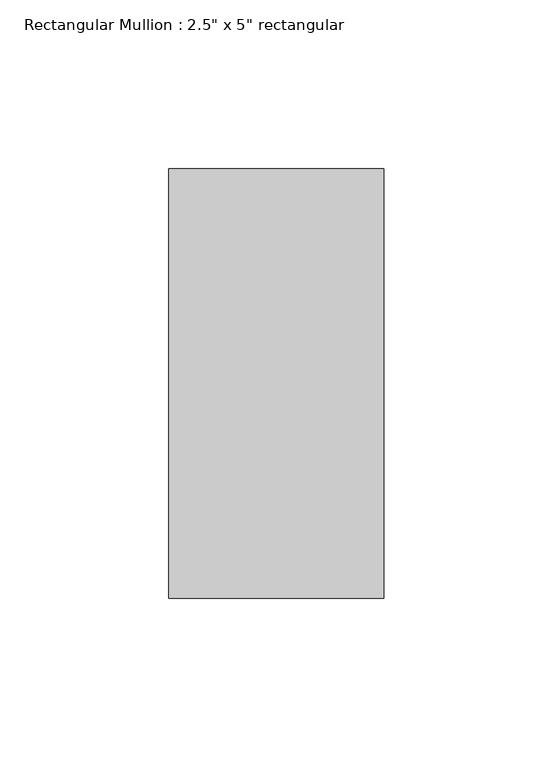
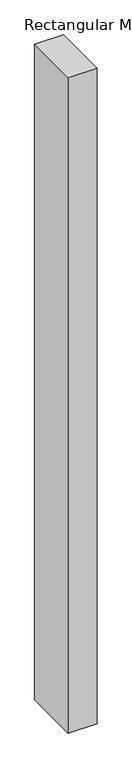
"""IFC4 building model written with IfcOpenShell, lengths in millimetres: member geometry."""

from ifc_helpers import new_model, si_unit, frame, origin, place, context, project, spatial, polyline, outline, extrude, source, transform, mapped, element, save


def member_82905deb(model_context):
    return source(origin(), model_context, "Body", "SweptSolid", [
        extrude(outline(polyline([(31.75, 63.5), (31.75, -63.5), (-31.75, -63.5), (-31.75, 63.5), (31.75, 63.5)])), frame((0.0, 0.0, -1524.0), z_axis=(0.0, 0.0, 1.0), x_axis=(1.0, 0.0, 0.0)), (0.0, 0.0, 1.0), 1524.0),
    ])


if __name__ == "__main__":
    model = new_model("IFC4")
    model_context = context("Model", 3, world=origin())
    ifc_project = project(units=[si_unit("LENGTHUNIT", "METRE", prefix="MILLI")], contexts=[model_context])
    site = spatial("IfcSite", under=ifc_project)
    building = spatial("IfcBuilding", under=site)
    placement = place(None, origin())
    member_shape = member_82905deb(model_context)
    element("IfcMember", 1, ObjectType="Rectangular Mullion : 2.5\" x 5\" rectangular", at=placement, inside=building, context=model_context, shape_type="MappedRepresentation", body=[
        mapped(member_shape, transform((0.0, 0.0, 0.0), x_axis=(1.0, 0.0, 0.0), y_axis=(0.0, 1.0, 0.0), z_axis=(0.0, 0.0, 1.0))),
    ])
    save(model, "model.ifc")

# Revit data of these elements
# Type "Rectangular Mullion : 2.5\" x 5\" rectangular"
#   built-in parameter 1007304 = 0.416667 (stored number, unit not read)
#   built-in parameter 1007301 = 0.104167 (stored number, unit not read)
#   built-in parameter 1007300 = 0.104167 (stored number, unit not read)
